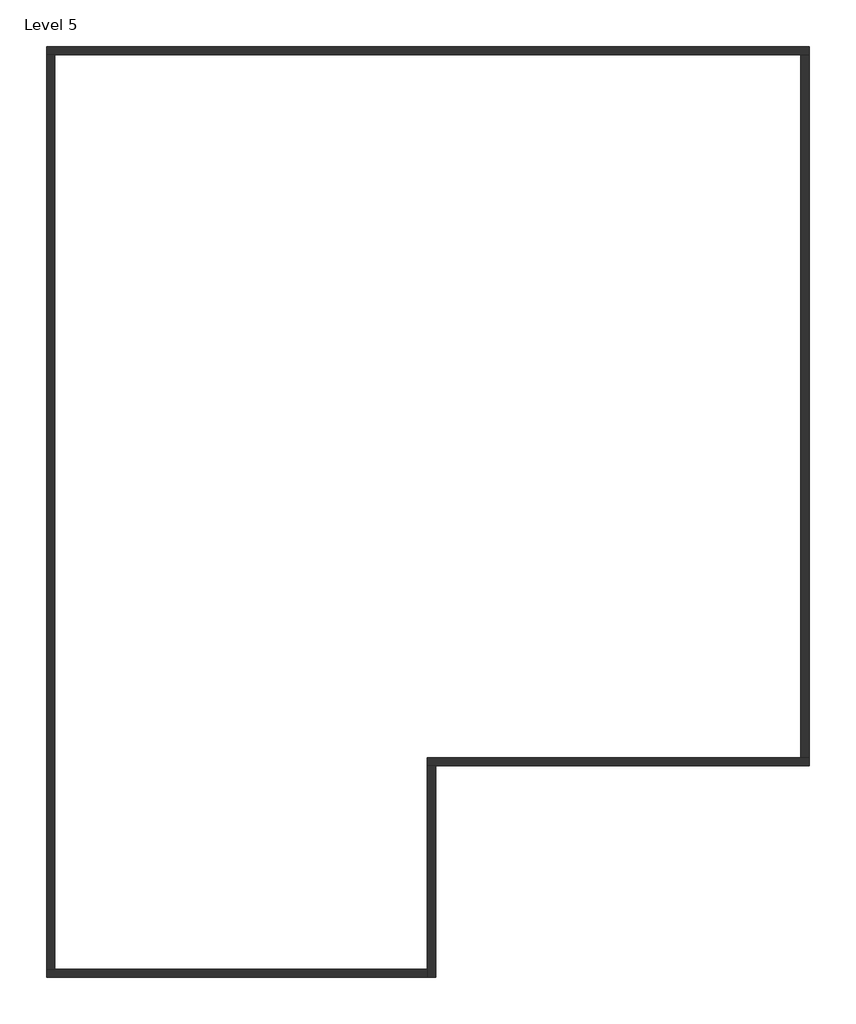
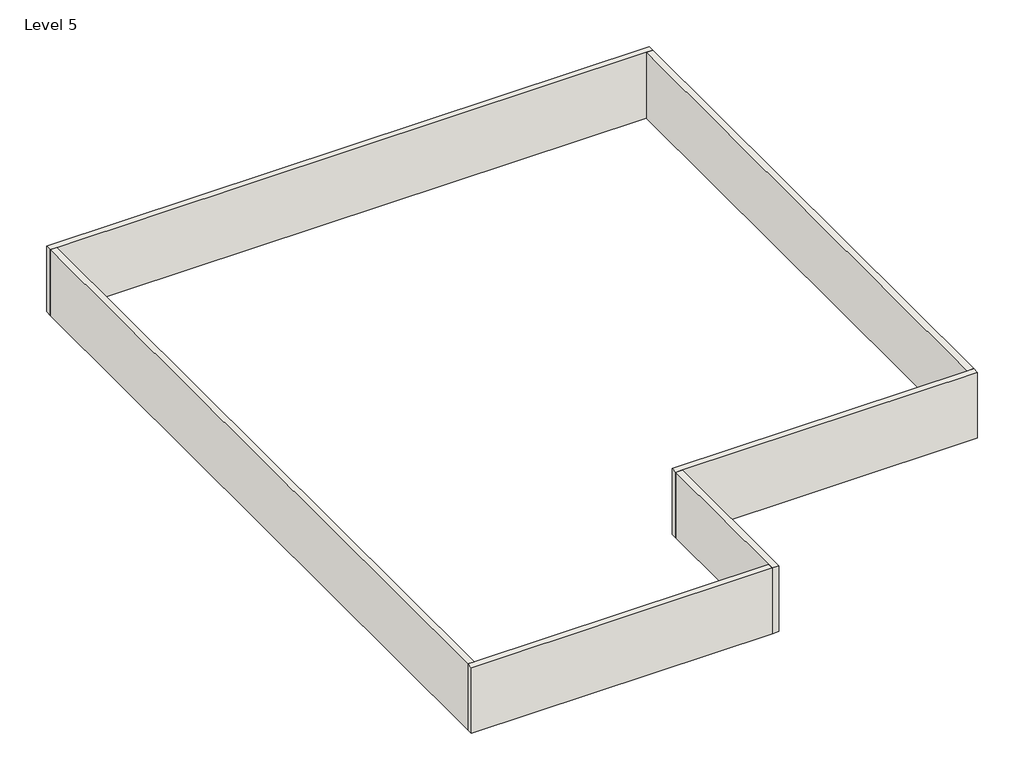
# One storey: 6 walls.
"""IFC4 building model written with IfcOpenShell, lengths in millimetres."""

from ifc_helpers import new_model, si_unit, frame, origin, place, context, project, spatial, polyline, outline, extrude, faceted_brep, element, save

model = new_model("IFC4")

# Units and contexts
model_context = context("Model", 3, world=origin())
ifc_project = project(units=[si_unit("LENGTHUNIT", "METRE", prefix="MILLI")], contexts=[model_context])

# Site, building, storey
site = spatial("IfcSite", under=ifc_project)
building = spatial("IfcBuilding", under=site)
storey = spatial("IfcBuildingStorey", under=building, Name="Level 5", Elevation=7010.4)

# Walls
placement = place(None, origin())
element("IfcWall", 1, ObjectType="4.5\" wall", at=placement, inside=storey, context=model_context, shape_type="Brep", body=[
    faceted_brep([(793.8459691, 3243.2033856, 7010.4), (679.5459691, 3243.2033856, 7010.4), (-4502.0540309, 3243.2033856, 7010.4), (-4502.0540309, 3243.2033856, 8229.6), (679.5459691, 3243.2033856, 8229.6), (793.8459691, 3243.2033856, 8229.6), (793.8459691, 3128.9033856, 7010.4), (793.8459691, 3128.9033856, 8229.6), (-4387.7540309, 3128.9033856, 8229.6), (-4502.0540309, 3128.9033856, 8229.6), (-4502.0540309, 3128.9033856, 7010.4), (-4387.7540309, 3128.9033856, 7010.4)], [[[0, 1, 2, 3, 4, 5]], [[6, 7, 8, 9, 10, 11]], [[2, 1, 0, 6, 11, 10]], [[5, 4, 3, 9, 8, 7]], [[3, 2, 10, 9]], [[0, 5, 7, 6]]]),
])
element("IfcWall", 2, ObjectType="4.5\" wall", at=placement, inside=storey, context=model_context, shape_type="Brep", body=[
    faceted_brep([(-4502.0540309, 3128.9033856, 7010.4), (-4502.0540309, 309.5033856, 7010.4), (-4502.0540309, 195.2033856, 7010.4), (-4502.0540309, 195.2033856, 8229.6), (-4502.0540309, 309.5033856, 8229.6), (-4502.0540309, 3128.9033856, 8229.6), (-4387.7540309, 3128.9033856, 7010.4), (-4387.7540309, 3128.9033856, 8229.6), (-4387.7540309, 195.2033856, 8229.6), (-4387.7540309, 195.2033856, 7010.4)], [[[0, 1, 2, 3, 4, 5]], [[6, 7, 8, 9]], [[2, 1, 0, 6, 9]], [[5, 4, 3, 8, 7]], [[0, 5, 7, 6]], [[3, 2, 9, 8]]]),
])
element("IfcWall", 3, ObjectType="4.5\" wall", at=placement, inside=storey, context=model_context, shape_type="Brep", body=[
    faceted_brep([(-4502.0540309, 309.5033856, 7010.4), (-9670.9540309, 309.5033856, 7010.4), (-9785.2540309, 309.5033856, 7010.4), (-9785.2540309, 309.5033856, 8229.6), (-9670.9540309, 309.5033856, 8229.6), (-4502.0540309, 309.5033856, 8229.6), (-4502.0540309, 195.2033856, 7010.4), (-4502.0540309, 195.2033856, 8229.6), (-9785.2540309, 195.2033856, 8229.6), (-9785.2540309, 195.2033856, 7010.4)], [[[0, 1, 2, 3, 4, 5]], [[6, 7, 8, 9]], [[2, 1, 0, 6, 9]], [[5, 4, 3, 8, 7]], [[0, 5, 7, 6]], [[3, 2, 9, 8]]]),
])
element("IfcWall", 4, ObjectType="4.5\" wall", at=placement, inside=storey, context=model_context, shape_type="Brep", body=[
    faceted_brep([(-9785.2540309, 12996.8033856, 7010.4), (-9670.9540309, 12996.8033856, 7010.4), (679.5459691, 12996.8033856, 7010.4), (793.8459691, 12996.8033856, 7010.4), (793.8459691, 12996.8033856, 8229.6), (679.5459691, 12996.8033856, 8229.6), (-9670.9540309, 12996.8033856, 8229.6), (-9785.2540309, 12996.8033856, 8229.6), (-9785.2540309, 13111.1033856, 7010.4), (-9785.2540309, 13111.1033856, 8229.6), (793.8459691, 13111.1033856, 8229.6), (793.8459691, 13111.1033856, 7010.4)], [[[0, 1, 2, 3, 4, 5, 6, 7]], [[8, 9, 10, 11]], [[3, 2, 1, 0, 8, 11]], [[7, 6, 5, 4, 10, 9]], [[4, 3, 11, 10]], [[0, 7, 9, 8]]]),
])
element("IfcWall", 5, ObjectType="4.5\" wall", at=placement, inside=storey, context=model_context, shape_type="SweptSolid", body=[
    extrude(outline(polyline([(679.5459691, 3243.2033856), (679.5459691, 12996.8033856), (793.8459691, 12996.8033856), (793.8459691, 3243.2033856), (679.5459691, 3243.2033856)])), frame((0.0, 0.0, 7010.4), z_axis=(0.0, 0.0, 1.0), x_axis=(1.0, 0.0, 0.0)), (0.0, 0.0, 1.0), 1219.2),
])
element("IfcWall", 6, ObjectType="4.5\" wall", at=placement, inside=storey, context=model_context, shape_type="SweptSolid", body=[
    extrude(outline(polyline([(-9785.2540309, 309.5033856), (-9785.2540309, 12996.8033856), (-9670.9540309, 12996.8033856), (-9670.9540309, 309.5033856), (-9785.2540309, 309.5033856)])), frame((0.0, 0.0, 7010.4), z_axis=(0.0, 0.0, 1.0), x_axis=(1.0, 0.0, 0.0)), (0.0, 0.0, 1.0), 1219.2),
])

save(model, "model.ifc")

# Revit data of these elements
# Type "4.5\" wall"
#   Assembly Code = "B2010"
#   Layers, outside or top first: 0' - 4 1/2" "Gypsum Wall Board" (function 1)
# Elements 1, 2, 3, 4, 5, 6 (IfcWall, "4.5\" wall")
#   Top Offset = 0' - 0"
#   Base Offset = 0' - 0"
#   wall height = 4' - 0"
#   Phase Created = New Construction
#   Base Constraint = Level 5
#   Top Constraint = Level 6
#   Materials on its faces: "Gypsum Wall Board"
# Materials
#   "Gypsum Wall Board": class "Generic", colour RGB 127 127 127, transparency 0, Description = "Gypsum Wall Board", Cost = 0
